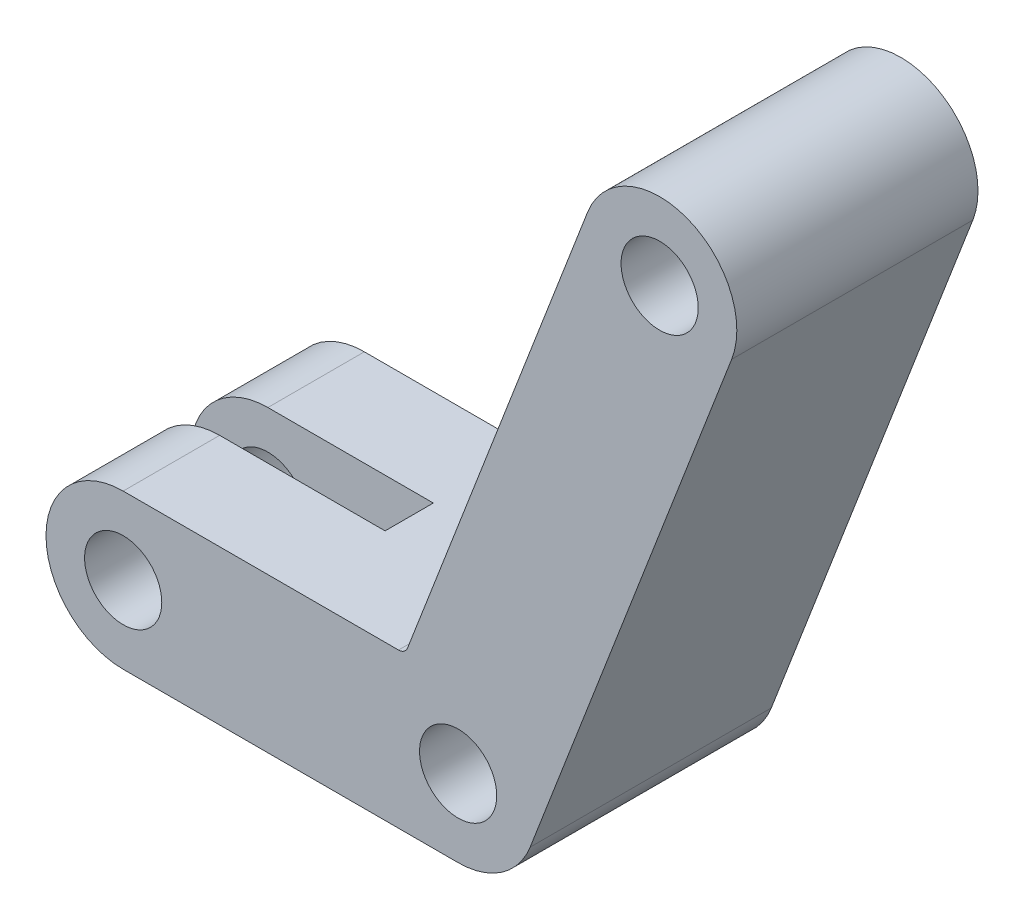
SolidWorks part; units mm, degrees
material "Plain Carbon Steel"
ref_plane "Front Plane" through (0, 0, 0) normal (0, 0, 1) x (1, 0, 0)
ref_plane "Top Plane" through (0, 0, 0) normal (0, 1, 0) x (1, 0, 0)
ref_plane "Right Plane" through (0, 0, 0) normal (1, 0, 0) x (0, 0, -1)
sketch "Jaw Profile Sketch" plane through (0, 0, 0) normal (0, 0, 1) x (1, 0, 0)
  line L0 (17.36, 0) -> (-17.36, 0) construction
  line L1 (17.36, -8) -> (-17.36, -8)
  line L2 (11.8683, 8) -> (-17.36, 8)
  line L3 (17.36, 0) -> (38.25, 54.24) construction
  line L4 (11.8683, 8) -> (30.7845, 57.1152)
  line L5 (24.8255, -2.8752) -> (45.7155, 51.3648)
  arc A0 (17.36, -8) -> (24.8255, -2.8752) centre (17.36, 0) ccw
  arc A1 (-17.36, 8) -> (-17.36, -8) centre (-17.36, 0) ccw
  arc A3 (45.7155, 51.3648) -> (30.7845, 57.1152) centre (38.25, 54.24) ccw
  arc A4 (17.36, -8) -> (24.8255, -2.8752) centre (17.36, 0) ccw
  circle A5 centre (17.36, 0) radius 4
  circle A6 centre (-17.36, 0) radius 4
  circle A7 centre (38.25, 54.24) radius 4
  point P2 (0, 0)
  point P10 (27.805, 27.12)
  dimension "D2" = 8
  dimension "D6" = 8
  dimension "D1" = 34.72
  dimension "D3" = 54.24
  dimension "D4" = 20.89
extrude "Jaw Body 25mm" add sketch "Jaw Profile Sketch" along normal mid plane 25 contours L5 A3 L4 L2 A1 L1 A0 A7 A6 A5
sketch "Slot Sketch" plane through (0, 8, 0) normal (0, 1, 0) x (1, 0, 0)
  line L0 (-25.36, 12.5) -> (-25.36, -12.5) construction
  line L1 (-0.21, -2.5) -> (-25.36, -2.5)
  line L2 (-0.21, -2.5) -> (-0.21, 2.5)
  line L3 (-0.21, 2.5) -> (-25.36, 2.5)
  line L4 (-25.36, -2.5) -> (-25.36, 2.5)
  line L5 (-0.21, -2.5) -> (-25.36, 2.5) construction
  line L6 (-0.21, 2.5) -> (-25.36, -2.5) construction
  point P0 (-12.785, 0)
  point P7 (-0.21, 0)
  dimension "D1" = 5
  dimension "D2" = 25.15
extrude "Slot Cut 5mm" cut sketch "Slot Sketch" against normal blind 25
fillet "Edge Fillets R1" radius 1 1 edges at (11.8683, 8, 0)
